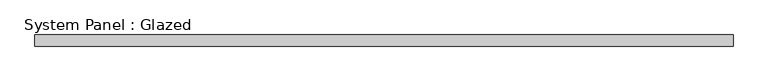
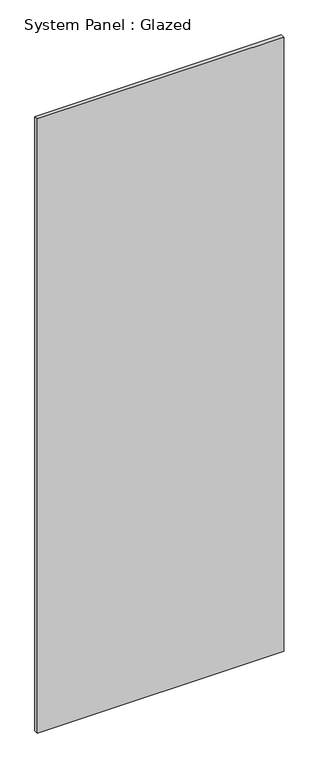
"""IFC4 building model written with IfcOpenShell, lengths in millimetres: plate geometry, System Panel : Glazed."""

from ifc_helpers import new_model, si_unit, origin, origin_with_axes, place, context, project, spatial, polyline, outline, extrude, source, transform, mapped, element, save


def system_panel_glazed_533a1375(model_context):
    return source(origin(), model_context, "Body", "SweptSolid", [
        extrude(outline(polyline([(759.2989957, 24.5), (-759.2989957, 24.5), (-759.2989957, 49.5), (759.2989957, 49.5), (759.2989957, 24.5)])), origin_with_axes(), (0.0, 0.0, 1.0), 4000.0),
    ])


if __name__ == "__main__":
    model = new_model("IFC4")
    model_context = context("Model", 3, world=origin())
    ifc_project = project(units=[si_unit("LENGTHUNIT", "METRE", prefix="MILLI")], contexts=[model_context])
    site = spatial("IfcSite", under=ifc_project)
    building = spatial("IfcBuilding", under=site)
    placement = place(None, origin())
    system_panel_glazed_shape = system_panel_glazed_533a1375(model_context)
    element("IfcPlate", 1, ObjectType="System Panel : Glazed", at=placement, inside=building, context=model_context, shape_type="MappedRepresentation", body=[
        mapped(system_panel_glazed_shape, transform((0.0, 0.0, 0.0), x_axis=(1.0, 0.0, 0.0), y_axis=(0.0, 1.0, 0.0), z_axis=(0.0, 0.0, 1.0))),
    ])
    save(model, "model.ifc")

# Revit data of these elements
# Type "System Panel : Glazed"
#   Keynote = "H11"
#   Construction Type Id = "GSP4R"
#   Analytic Construction = "1/8 in Pilkington single glazing"
#   Visual Light Transmittance = 0.9
#   Solar Heat Gain Coefficient = 0.86
#   Heat Transfer Coefficient (U) = 6.7069 W/(m²·K)
#   Define Thermal Properties by = 1
# Element 1 (IfcPlate, "System Panel : Glazed")
#   Materials on its faces: "Glass"
# Materials
#   "Glass": class "Glass", colour RGB 0 128 192, transparency 0.9, Description = "Soda Lime Glass", Cost = 0
